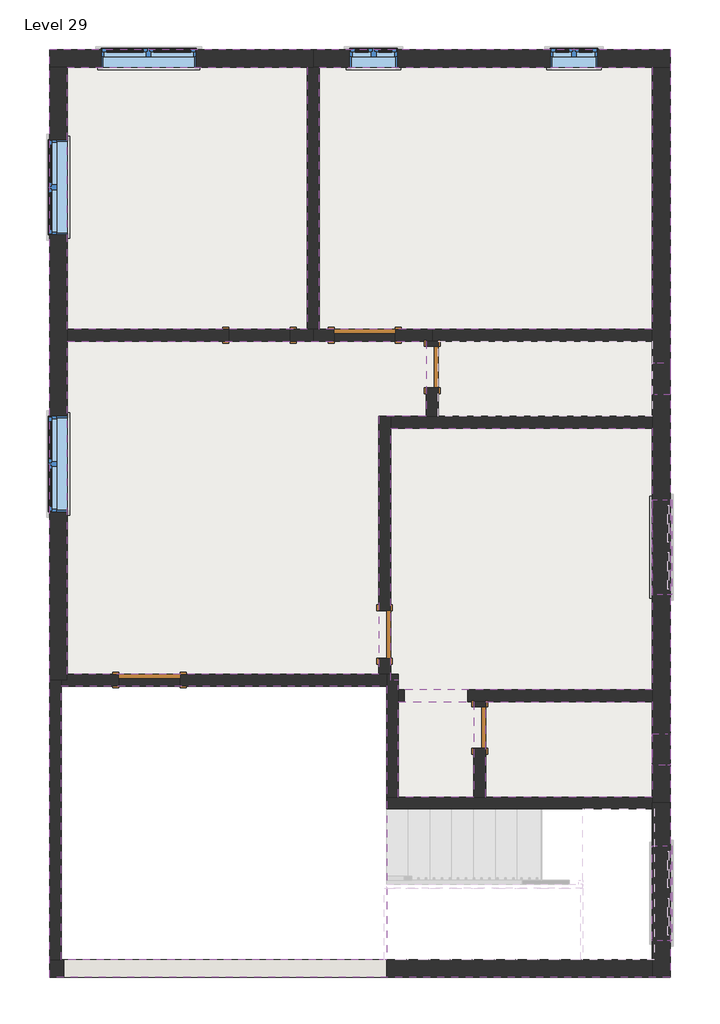
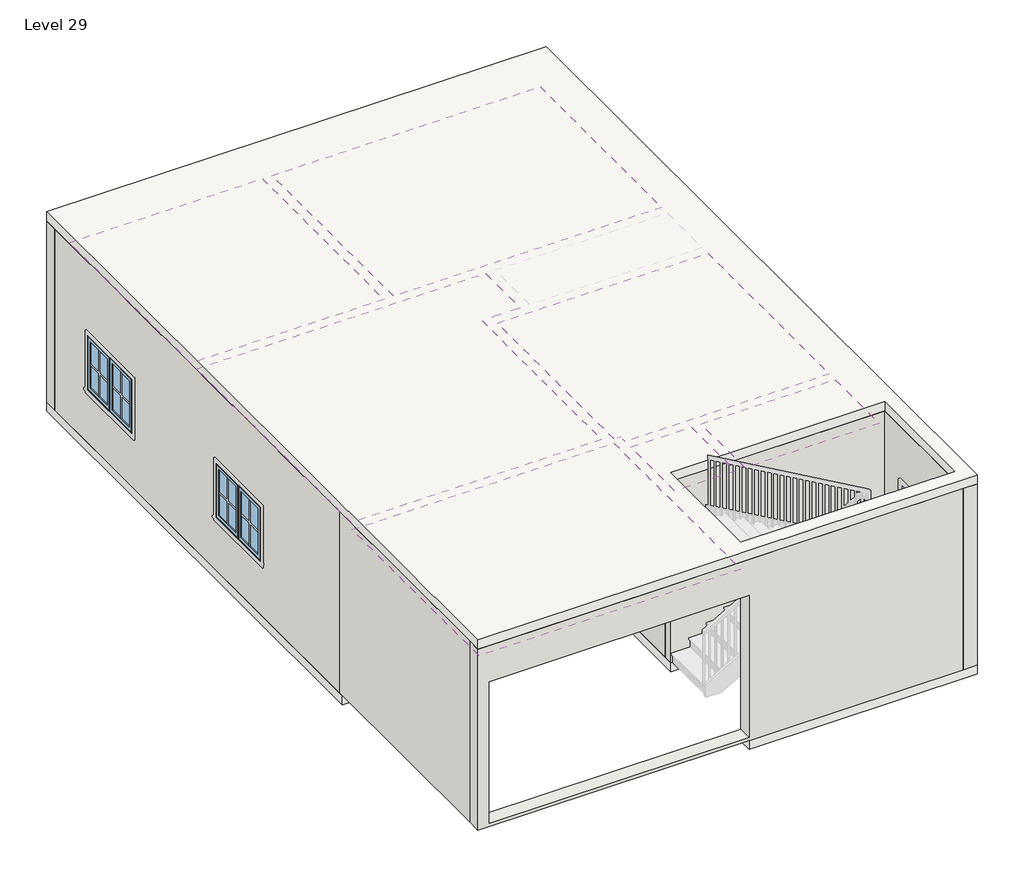
# One storey, part 1 of 2: 27 walls, 13 windows, 7 coverings, 6 doors, 2 slabs.
"""IFC4 building model written with IfcOpenShell, lengths in millimetres."""

from ifc_helpers import new_model, si_unit, frame, origin, place, context, project, spatial, polyline, outline, extrude, faceted_brep, transform, mapped, element, save
from components import door_2908be75, door_9ea4ff49, door_dc34e247, door_b804d09e, fixed_2_415b3208, window_casement_double_3_c417fced, window_casement_double_4_c19c33cb

model = new_model("IFC4")

# Units and contexts
model_context = context("Model", 3, world=origin())
ifc_project = project(units=[si_unit("LENGTHUNIT", "METRE", prefix="MILLI")], contexts=[model_context])

# Site, building, storey
site = spatial("IfcSite", under=ifc_project)
building = spatial("IfcBuilding", under=site)
storey = spatial("IfcBuildingStorey", under=building, Name="Level 29", Elevation=25603.2)

# Coverings
placement = place(None, origin())
element("IfcCovering", 1, ObjectType="2' x 4' ACT System", at=placement, inside=storey, context=model_context, shape_type="SweptSolid", body=[
    extrude(outline(polyline([(-5680.5154463, 2323.8455275), (-5680.5154463, 5678.2330275), (-2607.1154463, 5678.2330275), (-2607.1154463, 2323.8455275), (-5680.5154463, 2323.8455275)])), frame((0.0, 0.0, 28346.4), z_axis=(0.0, 0.0, 1.0), x_axis=(1.0, 0.0, 0.0)), (0.0, 0.0, 1.0), 57.15),
])
element("IfcCovering", 2, ObjectType="2' x 4' ACT System", at=placement, inside=storey, context=model_context, shape_type="SweptSolid", body=[
    extrude(outline(polyline([(-2454.7154463, 2323.8455275), (-2454.7154463, 5678.2330275), (1812.4845537, 5678.2330275), (1812.4845537, 2323.8455275), (-2454.7154463, 2323.8455275)])), frame((0.0, 0.0, 28346.4), z_axis=(0.0, 0.0, 1.0), x_axis=(1.0, 0.0, 0.0)), (0.0, 0.0, 1.0), 57.15),
])
element("IfcCovering", 3, ObjectType="2' x 4' ACT System", at=placement, inside=storey, context=model_context, shape_type="SweptSolid", body=[
    extrude(outline(polyline([(-5680.5154463, -2095.7544725), (-5680.5154463, 2171.4455275), (-1083.1154463, 2171.4455275), (-1083.1154463, 1206.2455275), (-1692.7154463, 1206.2455275), (-1692.7154463, -2095.7544725), (-5680.5154463, -2095.7544725)])), frame((0.0, 0.0, 28346.4), z_axis=(0.0, 0.0, 1.0), x_axis=(1.0, 0.0, 0.0)), (0.0, 0.0, 1.0), 57.15),
])
element("IfcCovering", 4, ObjectType="2' x 4' ACT System", at=placement, inside=storey, context=model_context, shape_type="SweptSolid", body=[
    extrude(outline(polyline([(1812.4845537, 1053.8455275), (1812.4845537, -2298.9544725), (-1438.7154463, -2298.9544725), (-1438.7154463, -2171.9544725), (-1540.3154463, -2171.9544725), (-1540.3154463, 1053.8455275), (1812.4845537, 1053.8455275)])), frame((0.0, 0.0, 28346.4), z_axis=(0.0, 0.0, 1.0), x_axis=(1.0, 0.0, 0.0)), (0.0, 0.0, 1.0), 57.15),
])
element("IfcCovering", 5, ObjectType="2' x 4' ACT System", at=placement, inside=storey, context=model_context, shape_type="SweptSolid", body=[
    extrude(outline(polyline([(1812.4845537, -2451.3544725), (1812.4845537, -3670.5544725), (-321.1154463, -3670.5544725), (-321.1154463, -2451.3544725), (1812.4845537, -2451.3544725)])), frame((0.0, 0.0, 28346.4), z_axis=(0.0, 0.0, 1.0), x_axis=(1.0, 0.0, 0.0)), (0.0, 0.0, 1.0), 57.15),
])
element("IfcCovering", 6, ObjectType="2' x 4' ACT System", at=placement, inside=storey, context=model_context, shape_type="SweptSolid", body=[
    extrude(outline(polyline([(-473.5154463, -2451.3544725), (-473.5154463, -3670.5544725), (-1438.7154463, -3670.5544725), (-1438.7154463, -2451.3544725), (-473.5154463, -2451.3544725)])), frame((0.0, 0.0, 28346.4), z_axis=(0.0, 0.0, 1.0), x_axis=(1.0, 0.0, 0.0)), (0.0, 0.0, 1.0), 57.15),
])
element("IfcCovering", 7, ObjectType="2' x 4' ACT System", at=placement, inside=storey, context=model_context, shape_type="SweptSolid", body=[
    extrude(outline(polyline([(-1591.1154463, -2248.1544725), (-1591.1154463, -5753.3544725), (-5756.7154463, -5753.3544725), (-5756.7154463, -2248.1544725), (-1591.1154463, -2248.1544725)])), frame((0.0, 0.0, 28346.4), z_axis=(0.0, 0.0, 1.0), x_axis=(1.0, 0.0, 0.0)), (0.0, 0.0, 1.0), 57.15),
])

# Doors
door_shape = door_2908be75(model_context)
element("IfcDoor", 8, ObjectType="Single-Flush : 1' 9\"", at=placement, inside=storey, context=model_context, shape_type="MappedRepresentation", body=[
    mapped(door_shape, transform((-397.3154463, -2781.5544725, 25603.2), x_axis=(0.0, 1.0, 0.0), y_axis=(-1.0, 0.0, 0.0), z_axis=(0.0, 0.0, 1.0))),
])
element("IfcDoor", 9, ObjectType="Single-Flush : 1' 9\"", at=placement, inside=storey, context=model_context, shape_type="MappedRepresentation", body=[
    mapped(door_shape, transform((-1006.9154463, 1841.2455275, 25603.2), x_axis=(0.0, 1.0, 0.0), y_axis=(-1.0, 0.0, 0.0), z_axis=(0.0, 0.0, 1.0))),
])
door_2_shape = door_9ea4ff49(model_context)
element("IfcDoor", 10, ObjectType="Single-Flush : 2'0\"", at=placement, inside=storey, context=model_context, shape_type="MappedRepresentation", body=[
    mapped(door_2_shape, transform((-1616.5154463, -1587.7544725, 25603.2), x_axis=(0.0, -1.0, 0.0), y_axis=(1.0, 0.0, 0.0), z_axis=(0.0, 0.0, 1.0))),
])
door_3_shape = door_dc34e247(model_context)
element("IfcDoor", 11, ObjectType="Single-Flush : 2'7\"", at=placement, inside=storey, context=model_context, shape_type="MappedRepresentation", body=[
    mapped(door_3_shape, transform((-4626.4154463, -2171.9544725, 25603.2), x_axis=(-1.0, 0.0, 0.0), y_axis=(0.0, -1.0, 0.0), z_axis=(0.0, 0.0, 1.0))),
])
element("IfcDoor", 12, ObjectType="Single-Flush : 2'7\"", at=placement, inside=storey, context=model_context, shape_type="MappedRepresentation", body=[
    mapped(door_3_shape, transform((-1870.5154463, 2247.6455275, 25603.2), x_axis=(-1.0, 0.0, 0.0), y_axis=(0.0, -1.0, 0.0), z_axis=(0.0, 0.0, 1.0))),
])
door_4_shape = door_b804d09e(model_context)
element("IfcDoor", 13, ObjectType="Single-Flush : 2'7\"", at=placement, inside=storey, context=model_context, shape_type="MappedRepresentation", body=[
    mapped(door_4_shape, transform((-3216.7154463, 2247.6455275, 25603.2), x_axis=(1.0, 0.0, 0.0), y_axis=(0.0, 1.0, 0.0), z_axis=(0.0, 0.0, 1.0))),
])

# Slabs
element("IfcSlab", 14, ObjectType="Generic - 6\"", at=placement, inside=storey, context=model_context, shape_type="SweptSolid", body=[
    extrude(outline(polyline([(-5909.1154463, -2248.1544725), (-5909.1154463, 5906.8330275), (2041.0845537, 5906.8330275), (2041.0845537, -5981.9544725), (-1591.1154463, -5981.9544725), (-1591.1154463, -5753.3544725), (1812.4845537, -5753.3544725), (1812.4845537, -3822.9544725), (-1591.1154463, -3822.9544725), (-1591.1154463, -2248.1544725), (-5756.7154463, -2248.1544725), (-5909.1154463, -2248.1544725)])), frame((0.0, 0.0, 25450.8), z_axis=(0.0, 0.0, 1.0), x_axis=(1.0, 0.0, 0.0)), (0.0, 0.0, 1.0), 152.4),
])
element("IfcSlab", 15, ObjectType="Generic - 6\"", at=placement, inside=storey, context=model_context, shape_type="SweptSolid", body=[
    extrude(outline(polyline([(2041.0845537, 5906.8330275), (2041.0845537, -5981.9544725), (-5909.1154463, -5981.9544725), (-5909.1154463, 5906.8330275), (2041.0845537, 5906.8330275)]), holes=[polyline([(1812.4845537, -3822.9544725), (-1591.1154463, -3822.9544725), (-1591.1154463, -5753.3544725), (1812.4845537, -5753.3544725), (1812.4845537, -3822.9544725)])]), frame((0.0, 0.0, 28651.2), z_axis=(0.0, 0.0, 1.0), x_axis=(1.0, 0.0, 0.0)), (0.0, 0.0, 1.0), 152.4),
])

# Walls
element("IfcWall", 16, ObjectType="Generic - 6\"", at=placement, inside=storey, context=model_context, shape_type="Brep", body=[
    faceted_brep([(-5909.1154463, -2171.9544725, 25603.2), (-5909.1154463, -5753.3544725, 25603.2), (-5909.1154463, -5753.3544725, 28651.2), (-5909.1154463, -2171.9544725, 28651.2), (-5756.7154463, -2171.9544725, 25603.2), (-5756.7154463, -2171.9544725, 28651.2), (-5756.7154463, -2248.1544725, 28651.2), (-5756.7154463, -5753.3544725, 28651.2), (-5756.7154463, -5753.3544725, 25603.2), (-5756.7154463, -2248.1544725, 25603.2)], [[[0, 1, 2, 3]], [[4, 5, 6, 7, 8, 9]], [[1, 0, 4, 9, 8]], [[3, 2, 7, 6, 5]], [[0, 3, 5, 4]], [[2, 1, 8, 7]]]),
])
element("IfcWall", 17, ObjectType="Generic - 6\"", at=placement, inside=storey, context=model_context, shape_type="Brep", body=[
    faceted_brep([(1812.4845537, -3670.5544725, 25603.2), (-321.1154463, -3670.5544725, 25603.2), (-473.5154463, -3670.5544725, 25603.2), (-1438.7154463, -3670.5544725, 25603.2), (-1591.1154463, -3670.5544725, 25603.2), (-1591.1154463, -3670.5544725, 28651.2), (-1438.7154463, -3670.5544725, 28651.2), (-473.5154463, -3670.5544725, 28651.2), (-321.1154463, -3670.5544725, 28651.2), (1812.4845537, -3670.5544725, 28651.2), (1812.4845537, -3822.9544725, 25603.2), (1812.4845537, -3822.9544725, 28651.2), (-1591.1154463, -3822.9544725, 28651.2), (-1591.1154463, -3822.9544725, 25603.2), (1812.4845537, -3746.7544725, 25603.2), (1812.4845537, -3746.7544725, 28651.2)], [[[0, 1, 2, 3, 4, 5, 6, 7, 8, 9]], [[10, 11, 12, 13]], [[4, 3, 2, 1, 0, 14, 10, 13]], [[9, 8, 7, 6, 5, 12, 11, 15]], [[5, 4, 13, 12]], [[0, 9, 15, 11, 10, 14]]]),
])
element("IfcWall", 18, ObjectType="Generic - 6\"", at=placement, inside=storey, context=model_context, shape_type="Brep", body=[
    faceted_brep([(-1438.7154463, -3670.5544725, 25603.2), (-1438.7154463, -2451.3544725, 25603.2), (-1438.7154463, -2298.9544725, 25603.2), (-1438.7154463, -2095.7544725, 25603.2), (-1438.7154463, -2095.7544725, 28651.2), (-1438.7154463, -2298.9544725, 28651.2), (-1438.7154463, -2451.3544725, 28651.2), (-1438.7154463, -3670.5544725, 28651.2), (-1591.1154463, -3670.5544725, 25603.2), (-1591.1154463, -3670.5544725, 28651.2), (-1591.1154463, -2248.1544725, 28651.2), (-1591.1154463, -2171.9544725, 28651.2), (-1591.1154463, -2095.7544725, 28651.2), (-1591.1154463, -2095.7544725, 25603.2), (-1591.1154463, -2171.9544725, 25603.2), (-1591.1154463, -2248.1544725, 25603.2), (-1540.3154463, -2095.7544725, 25603.2), (-1540.3154463, -2095.7544725, 28651.2)], [[[0, 1, 2, 3, 4, 5, 6, 7]], [[8, 9, 10, 11, 12, 13, 14, 15]], [[3, 2, 1, 0, 8, 15, 14, 13, 16]], [[7, 6, 5, 4, 17, 12, 11, 10, 9]], [[0, 7, 9, 8]], [[4, 3, 16, 13, 12, 17]]]),
])
element("IfcWall", 19, ObjectType="Generic - 6\"", at=placement, inside=storey, context=model_context, shape_type="Brep", body=[
    faceted_brep([(-5020.1154463, -2095.7544725, 27736.8), (-5020.1154463, -2095.7544725, 25603.2), (-5680.5154463, -2095.7544725, 25603.2), (-5680.5154463, -2095.7544725, 28651.2), (-1692.7154463, -2095.7544725, 28651.2), (-1591.1154463, -2095.7544725, 28651.2), (-1591.1154463, -2095.7544725, 25603.2), (-1692.7154463, -2095.7544725, 25603.2), (-4232.7154463, -2095.7544725, 25603.2), (-4232.7154463, -2095.7544725, 27736.8), (-5756.7154463, -2248.1544725, 25603.2), (-5020.1154463, -2248.1544725, 25603.2), (-5020.1154463, -2248.1544725, 27736.8), (-4232.7154463, -2248.1544725, 27736.8), (-4232.7154463, -2248.1544725, 25603.2), (-1591.1154463, -2248.1544725, 25603.2), (-1591.1154463, -2248.1544725, 28651.2), (-5756.7154463, -2248.1544725, 28651.2), (-5756.7154463, -2171.9544725, 25603.2), (-5680.5154463, -2171.9544725, 25603.2), (-5680.5154463, -2171.9544725, 28651.2), (-5756.7154463, -2171.9544725, 28651.2)], [[[0, 1, 2, 3, 4, 5, 6, 7, 8, 9]], [[10, 11, 12, 13, 14, 15, 16, 17]], [[2, 1, 11, 10, 18, 19]], [[8, 7, 6, 15, 14]], [[5, 4, 3, 20, 21, 17, 16]], [[3, 2, 19, 20]], [[19, 18, 21, 20]], [[18, 10, 17, 21]], [[6, 5, 16, 15]], [[12, 11, 1, 0]], [[13, 12, 0, 9]], [[14, 13, 9, 8]]]),
])
element("IfcWall", 20, ObjectType="Generic - 6\"", at=placement, inside=storey, context=model_context, shape_type="Brep", body=[
    faceted_brep([(1812.4845537, -2451.3544725, 25603.2), (1812.4845537, -2451.3544725, 28651.2), (-321.1154463, -2451.3544725, 28651.2), (-473.5154463, -2451.3544725, 28651.2), (-1438.7154463, -2451.3544725, 28651.2), (-1438.7154463, -2451.3544725, 25603.2), (-1367.0206652, -2451.3544725, 25603.2), (-1367.0206652, -2451.3544725, 28041.6), (-547.4818767, -2451.3544725, 28041.6), (-547.4818767, -2451.3544725, 25603.2), (-473.5154463, -2451.3544725, 25603.2), (-321.1154463, -2451.3544725, 25603.2), (1812.4845537, -2298.9544725, 28651.2), (1812.4845537, -2298.9544725, 25603.2), (-547.4818767, -2298.9544725, 25603.2), (-547.4818767, -2298.9544725, 28041.6), (-1367.0206652, -2298.9544725, 28041.6), (-1367.0206652, -2298.9544725, 25603.2), (-1438.7154463, -2298.9544725, 25603.2), (-1438.7154463, -2298.9544725, 28651.2)], [[[0, 1, 2, 3, 4, 5, 6, 7, 8, 9, 10, 11]], [[12, 13, 14, 15, 16, 17, 18, 19]], [[5, 18, 17, 6]], [[13, 0, 11, 10, 9, 14]], [[4, 3, 2, 1, 12, 19]], [[1, 0, 13, 12]], [[5, 4, 19, 18]], [[7, 16, 15, 8]], [[16, 7, 6, 17]], [[8, 15, 14, 9]]]),
])
element("IfcWall", 21, ObjectType="Generic - 6\"", at=placement, inside=storey, context=model_context, shape_type="SweptSolid", body=[
    extrude(outline(polyline([(-2451.3544725, 25603.2), (-2514.8544725, 25603.2), (-2514.8544725, 27736.8), (-3048.2544725, 27736.8), (-3048.2544725, 25603.2), (-3670.5544725, 25603.2), (-3670.5544725, 28651.2), (-2451.3544725, 28651.2), (-2451.3544725, 25603.2)])), frame((-473.5154463, 0.0, 0.0), z_axis=(1.0, 0.0, 0.0), x_axis=(0.0, 1.0, 0.0)), (0.0, 0.0, 1.0), 152.4),
])
element("IfcWall", 22, ObjectType="Generic - 6\"", at=placement, inside=storey, context=model_context, shape_type="Brep", body=[
    faceted_brep([(-1540.3154463, -2095.7544725, 25603.2), (-1540.3154463, -1892.5544725, 25603.2), (-1540.3154463, -1892.5544725, 27736.8), (-1540.3154463, -1282.9544725, 27736.8), (-1540.3154463, -1282.9544725, 25603.2), (-1540.3154463, 1053.8455275, 25603.2), (-1540.3154463, 1206.2455275, 25603.2), (-1540.3154463, 1206.2455275, 28651.2), (-1540.3154463, 1053.8455275, 28651.2), (-1540.3154463, -2095.7544725, 28651.2), (-1692.7154463, -1892.5544725, 27736.8), (-1692.7154463, -1892.5544725, 25603.2), (-1692.7154463, -2095.7544725, 25603.2), (-1692.7154463, -2095.7544725, 28651.2), (-1692.7154463, 1206.2455275, 28651.2), (-1692.7154463, 1206.2455275, 25603.2), (-1692.7154463, -1282.9544725, 25603.2), (-1692.7154463, -1282.9544725, 27736.8), (-1591.1154463, -2095.7544725, 25603.2), (-1591.1154463, -2095.7544725, 28651.2)], [[[0, 1, 2, 3, 4, 5, 6, 7, 8, 9]], [[10, 11, 12, 13, 14, 15, 16, 17]], [[16, 15, 6, 5, 4]], [[12, 11, 1, 0, 18]], [[9, 8, 7, 14, 13, 19]], [[0, 9, 19, 13, 12, 18]], [[7, 6, 15, 14]], [[2, 1, 11, 10]], [[3, 2, 10, 17]], [[4, 3, 17, 16]]]),
])
element("IfcWall", 23, ObjectType="Generic - 6\"", at=placement, inside=storey, context=model_context, shape_type="Brep", body=[
    faceted_brep([(-1540.3154463, 1053.8455275, 25603.2), (1812.4845537, 1053.8455275, 25603.2), (1812.4845537, 1053.8455275, 28651.2), (-1540.3154463, 1053.8455275, 28651.2), (-1540.3154463, 1206.2455275, 25603.2), (-1540.3154463, 1206.2455275, 28651.2), (-1083.1154463, 1206.2455275, 28651.2), (-930.7154463, 1206.2455275, 28651.2), (1812.4845537, 1206.2455275, 28651.2), (1812.4845537, 1206.2455275, 25603.2), (-930.7154463, 1206.2455275, 25603.2), (-1083.1154463, 1206.2455275, 25603.2)], [[[0, 1, 2, 3]], [[4, 5, 6, 7, 8, 9, 10, 11]], [[1, 0, 4, 11, 10, 9]], [[3, 2, 8, 7, 6, 5]], [[0, 3, 5, 4]], [[2, 1, 9, 8]]]),
])
element("IfcWall", 24, ObjectType="Generic - 6\"", at=placement, inside=storey, context=model_context, shape_type="Brep", body=[
    faceted_brep([(-930.7154463, 2107.9455275, 27736.8), (-930.7154463, 2107.9455275, 25603.2), (-930.7154463, 2171.4455275, 25603.2), (-930.7154463, 2171.4455275, 28651.2), (-930.7154463, 1206.2455275, 28651.2), (-930.7154463, 1206.2455275, 25603.2), (-930.7154463, 1574.5455275, 25603.2), (-930.7154463, 1574.5455275, 27736.8), (-1083.1154463, 2171.4455275, 25603.2), (-1083.1154463, 2107.9455275, 25603.2), (-1083.1154463, 2107.9455275, 27736.8), (-1083.1154463, 1574.5455275, 27736.8), (-1083.1154463, 1574.5455275, 25603.2), (-1083.1154463, 1206.2455275, 25603.2), (-1083.1154463, 1206.2455275, 28651.2), (-1083.1154463, 2171.4455275, 28651.2), (-1006.9154463, 2171.4455275, 25603.2), (-1006.9154463, 2171.4455275, 28651.2)], [[[0, 1, 2, 3, 4, 5, 6, 7]], [[8, 9, 10, 11, 12, 13, 14, 15]], [[6, 5, 13, 12]], [[2, 1, 9, 8, 16]], [[4, 3, 17, 15, 14]], [[5, 4, 14, 13]], [[10, 9, 1, 0]], [[11, 10, 0, 7]], [[12, 11, 7, 6]], [[3, 2, 16, 8, 15, 17]]]),
])
element("IfcWall", 25, ObjectType="Generic - 6\"", at=placement, inside=storey, context=model_context, shape_type="Brep", body=[
    faceted_brep([(1812.4845537, 2323.8455275, 25603.2), (-1006.9154463, 2323.8455275, 25603.2), (-1006.9154463, 2323.8455275, 28651.2), (1812.4845537, 2323.8455275, 28651.2), (1812.4845537, 2171.4455275, 25603.2), (1812.4845537, 2171.4455275, 28651.2), (-930.7154463, 2171.4455275, 28651.2), (-1006.9154463, 2171.4455275, 28651.2), (-1006.9154463, 2171.4455275, 25603.2), (-930.7154463, 2171.4455275, 25603.2)], [[[0, 1, 2, 3]], [[4, 5, 6, 7, 8, 9]], [[1, 0, 4, 9, 8]], [[2, 1, 8, 7]], [[3, 2, 7, 6, 5]], [[0, 3, 5, 4]]]),
])
element("IfcWall", 26, ObjectType="Generic - 6\"", at=placement, inside=storey, context=model_context, shape_type="Brep", body=[
    faceted_brep([(-2607.1154463, 5678.2330275, 25603.2), (-2607.1154463, 2323.8455275, 25603.2), (-2607.1154463, 2323.8455275, 28651.2), (-2607.1154463, 5678.2330275, 28651.2), (-2454.7154463, 5678.2330275, 25603.2), (-2454.7154463, 5678.2330275, 28651.2), (-2454.7154463, 2323.8455275, 28651.2), (-2454.7154463, 2323.8455275, 25603.2), (-2530.9154463, 5678.2330275, 25603.2), (-2530.9154463, 2323.8455275, 25603.2), (-2530.9154463, 2323.8455275, 28651.2), (-2530.9154463, 5678.2330275, 28651.2)], [[[0, 1, 2, 3]], [[4, 5, 6, 7]], [[1, 0, 8, 4, 7, 9]], [[3, 2, 10, 6, 5, 11]], [[0, 3, 11, 5, 4, 8]], [[2, 1, 9, 7, 6, 10]]]),
])
element("IfcWall", 27, ObjectType="Generic - 6\"", at=placement, inside=storey, context=model_context, shape_type="Brep", body=[
    faceted_brep([(-2530.9154463, 2323.8455275, 25603.2), (-2607.1154463, 2323.8455275, 25603.2), (-2823.0154463, 2323.8455275, 25603.2), (-2823.0154463, 2323.8455275, 27736.8), (-3610.4154463, 2323.8455275, 27736.8), (-3610.4154463, 2323.8455275, 25603.2), (-5680.5154463, 2323.8455275, 25603.2), (-5680.5154463, 2323.8455275, 28651.2), (-2607.1154463, 2323.8455275, 28651.2), (-2530.9154463, 2323.8455275, 28651.2), (-2823.0154463, 2171.4455275, 27736.8), (-2823.0154463, 2171.4455275, 25603.2), (-2530.9154463, 2171.4455275, 25603.2), (-2530.9154463, 2171.4455275, 28651.2), (-5680.5154463, 2171.4455275, 28651.2), (-5680.5154463, 2171.4455275, 25603.2), (-3610.4154463, 2171.4455275, 25603.2), (-3610.4154463, 2171.4455275, 27736.8)], [[[0, 1, 2, 3, 4, 5, 6, 7, 8, 9]], [[10, 11, 12, 13, 14, 15, 16, 17]], [[16, 15, 6, 5]], [[12, 11, 2, 1, 0]], [[9, 8, 7, 14, 13]], [[0, 9, 13, 12]], [[7, 6, 15, 14]], [[5, 4, 17, 16]], [[4, 3, 10, 17]], [[3, 2, 11, 10]]]),
])
element("IfcWall", 28, ObjectType="Generic - 6\"", at=placement, inside=storey, context=model_context, shape_type="Brep", body=[
    faceted_brep([(-2264.2154463, 2323.8455275, 27736.8), (-2264.2154463, 2323.8455275, 25603.2), (-2454.7154463, 2323.8455275, 25603.2), (-2530.9154463, 2323.8455275, 25603.2), (-2530.9154463, 2323.8455275, 28651.2), (-2454.7154463, 2323.8455275, 28651.2), (-1006.9154463, 2323.8455275, 28651.2), (-1006.9154463, 2323.8455275, 25603.2), (-1476.8154463, 2323.8455275, 25603.2), (-1476.8154463, 2323.8455275, 27736.8), (-2530.9154463, 2171.4455275, 25603.2), (-2264.2154463, 2171.4455275, 25603.2), (-2264.2154463, 2171.4455275, 27736.8), (-1476.8154463, 2171.4455275, 27736.8), (-1476.8154463, 2171.4455275, 25603.2), (-1083.1154463, 2171.4455275, 25603.2), (-1006.9154463, 2171.4455275, 25603.2), (-1006.9154463, 2171.4455275, 28651.2), (-1083.1154463, 2171.4455275, 28651.2), (-2530.9154463, 2171.4455275, 28651.2)], [[[0, 1, 2, 3, 4, 5, 6, 7, 8, 9]], [[10, 11, 12, 13, 14, 15, 16, 17, 18, 19]], [[8, 7, 16, 15, 14]], [[3, 2, 1, 11, 10]], [[4, 3, 10, 19]], [[6, 5, 4, 19, 18, 17]], [[7, 6, 17, 16]], [[14, 13, 9, 8]], [[13, 12, 0, 9]], [[12, 11, 1, 0]]]),
])
element("IfcWall", 29, ObjectType="Generic - 6\"", at=placement, inside=storey, context=model_context, shape_type="SweptSolid", body=[
    extrude(outline(polyline([(-5680.5154463, -2095.7544725), (-1692.7154463, -2095.7544725), (-1692.7154463, -2171.9544725), (-1591.1154463, -2171.9544725), (-1591.1154463, -2248.1544725), (-5756.7154463, -2248.1544725), (-5756.7154463, -2171.9544725), (-5680.5154463, -2171.9544725), (-5680.5154463, -2095.7544725)])), frame((0.0, 0.0, 25603.2), z_axis=(0.0, 0.0, 1.0), x_axis=(1.0, 0.0, 0.0)), (0.0, 0.0, 1.0), 3048.0),
])
element("IfcWall", 30, ObjectType="Generic - 6\"", at=placement, inside=storey, context=model_context, shape_type="Brep", body=[
    faceted_brep([(-2607.1154463, 5678.2330275, 25603.2), (-2607.1154463, 2323.8455275, 25603.2), (-2607.1154463, 2323.8455275, 28651.2), (-2607.1154463, 5678.2330275, 28651.2), (-2454.7154463, 5678.2330275, 25603.2), (-2454.7154463, 5678.2330275, 28651.2), (-2454.7154463, 2323.8455275, 28651.2), (-2454.7154463, 2323.8455275, 25603.2), (-2530.9154463, 5678.2330275, 25603.2), (-2530.9154463, 2323.8455275, 25603.2), (-2530.9154463, 2323.8455275, 28651.2), (-2530.9154463, 5678.2330275, 28651.2)], [[[0, 1, 2, 3]], [[4, 5, 6, 7]], [[1, 0, 8, 4, 7, 9]], [[3, 2, 10, 6, 5, 11]], [[0, 3, 11, 5, 4, 8]], [[2, 1, 9, 7, 6, 10]]]),
])
element("IfcWall", 31, ObjectType="Generic - 6\"", at=placement, inside=storey, context=model_context, shape_type="Brep", body=[
    faceted_brep([(-2530.9154463, 2323.8455275, 25603.2), (-2607.1154463, 2323.8455275, 25603.2), (-5680.5154463, 2323.8455275, 25603.2), (-5680.5154463, 2323.8455275, 28651.2), (-2607.1154463, 2323.8455275, 28651.2), (-2530.9154463, 2323.8455275, 28651.2), (-2530.9154463, 2171.4455275, 25603.2), (-2530.9154463, 2171.4455275, 28651.2), (-5680.5154463, 2171.4455275, 28651.2), (-5680.5154463, 2171.4455275, 25603.2)], [[[0, 1, 2, 3, 4, 5]], [[6, 7, 8, 9]], [[2, 1, 0, 6, 9]], [[5, 4, 3, 8, 7]], [[0, 5, 7, 6]], [[3, 2, 9, 8]]]),
])
element("IfcWall", 32, ObjectType="Generic - 6\"", at=placement, inside=storey, context=model_context, shape_type="Brep", body=[
    faceted_brep([(-1006.9154463, 2323.8455275, 25603.2), (-2454.7154463, 2323.8455275, 25603.2), (-2530.9154463, 2323.8455275, 25603.2), (-2530.9154463, 2323.8455275, 28651.2), (-2454.7154463, 2323.8455275, 28651.2), (-1006.9154463, 2323.8455275, 28651.2), (-1006.9154463, 2171.4455275, 25603.2), (-1006.9154463, 2171.4455275, 28651.2), (-1083.1154463, 2171.4455275, 28651.2), (-2530.9154463, 2171.4455275, 28651.2), (-2530.9154463, 2171.4455275, 25603.2), (-1083.1154463, 2171.4455275, 25603.2)], [[[0, 1, 2, 3, 4, 5]], [[6, 7, 8, 9, 10, 11]], [[2, 1, 0, 6, 11, 10]], [[3, 2, 10, 9]], [[5, 4, 3, 9, 8, 7]], [[0, 5, 7, 6]]]),
])
element("IfcWall", 33, ObjectType="Generic - 9\"", at=placement, inside=storey, context=model_context, shape_type="Brep", body=[
    faceted_brep([(-5909.1154463, 5678.2330275, 25603.2), (-5680.5154463, 5678.2330275, 25603.2), (-2607.1154463, 5678.2330275, 25603.2), (-2530.9154463, 5678.2330275, 25603.2), (-2530.9154463, 5678.2330275, 28651.2), (-2607.1154463, 5678.2330275, 28651.2), (-5680.5154463, 5678.2330275, 28651.2), (-5909.1154463, 5678.2330275, 28651.2), (-4029.5154463, 5678.2330275, 27432.0), (-4029.5154463, 5678.2330275, 26517.6), (-5248.7154463, 5678.2330275, 26517.6), (-5248.7154463, 5678.2330275, 27432.0), (-5909.1154463, 5906.8330275, 25603.2), (-5909.1154463, 5906.8330275, 28651.2), (-2530.9154463, 5906.8330275, 28651.2), (-2530.9154463, 5906.8330275, 25603.2), (-4029.5154463, 5906.8330275, 27432.0), (-5248.7154463, 5906.8330275, 27432.0), (-5248.7154463, 5906.8330275, 26517.6), (-4029.5154463, 5906.8330275, 26517.6)], [[[0, 1, 2, 3, 4, 5, 6, 7], [8, 9, 10, 11]], [[12, 13, 14, 15], [16, 17, 18, 19]], [[3, 2, 1, 0, 12, 15]], [[4, 3, 15, 14]], [[7, 6, 5, 4, 14, 13]], [[0, 7, 13, 12]], [[9, 8, 16, 19]], [[10, 9, 19, 18]], [[11, 10, 18, 17]], [[8, 11, 17, 16]]]),
])
element("IfcWall", 34, ObjectType="Generic - 9\"", at=placement, inside=storey, context=model_context, shape_type="Brep", body=[
    faceted_brep([(1812.4845537, 5678.2330275, 25603.2), (1812.4845537, 2323.8455275, 25603.2), (1812.4845537, 2171.4455275, 25603.2), (1812.4845537, 1206.2455275, 25603.2), (1812.4845537, 1053.8455275, 25603.2), (1812.4845537, -2298.9544725, 25603.2), (1812.4845537, -2451.3544725, 25603.2), (1812.4845537, -3670.5544725, 25603.2), (1812.4845537, -3746.7544725, 25603.2), (1812.4845537, -3746.7544725, 28651.2), (1812.4845537, -3670.5544725, 28651.2), (1812.4845537, -2451.3544725, 28651.2), (1812.4845537, -2298.9544725, 28651.2), (1812.4845537, 1053.8455275, 28651.2), (1812.4845537, 1206.2455275, 28651.2), (1812.4845537, 2171.4455275, 28651.2), (1812.4845537, 2323.8455275, 28651.2), (1812.4845537, 5678.2330275, 28651.2), (1812.4845537, -1079.7544725, 27736.8), (1812.4845537, -1079.7544725, 26822.4), (1812.4845537, 139.4455275, 26822.4), (1812.4845537, 139.4455275, 27736.8), (1812.4845537, -3264.1544725, 28041.6), (1812.4845537, -3264.1544725, 27432.0), (1812.4845537, -2857.7544725, 27432.0), (1812.4845537, -2857.7544725, 28041.6), (1812.4845537, 1892.0455275, 28041.6), (1812.4845537, 1485.6455275, 28041.6), (1812.4845537, 1485.6455275, 27432.0), (1812.4845537, 1892.0455275, 27432.0), (2041.0845537, 5678.2330275, 25603.2), (2041.0845537, 5678.2330275, 28651.2), (2041.0845537, -3746.7544725, 28651.2), (2041.0845537, -3746.7544725, 25603.2), (2041.0845537, -1079.7544725, 27736.8), (2041.0845537, 139.4455275, 27736.8), (2041.0845537, 139.4455275, 26822.4), (2041.0845537, -1079.7544725, 26822.4), (2041.0845537, -3264.1544725, 28041.6), (2041.0845537, -2857.7544725, 28041.6), (2041.0845537, -2857.7544725, 27432.0), (2041.0845537, -3264.1544725, 27432.0), (2041.0845537, 1892.0455275, 28041.6), (2041.0845537, 1892.0455275, 27432.0), (2041.0845537, 1485.6455275, 27432.0), (2041.0845537, 1485.6455275, 28041.6)], [[[0, 1, 2, 3, 4, 5, 6, 7, 8, 9, 10, 11, 12, 13, 14, 15, 16, 17], [18, 19, 20, 21], [22, 23, 24, 25], [26, 27, 28, 29]], [[30, 31, 32, 33], [34, 35, 36, 37], [38, 39, 40, 41], [42, 43, 44, 45]], [[8, 7, 6, 5, 4, 3, 2, 1, 0, 30, 33]], [[9, 8, 33, 32]], [[17, 16, 15, 14, 13, 12, 11, 10, 9, 32, 31]], [[0, 17, 31, 30]], [[19, 18, 34, 37]], [[20, 19, 37, 36]], [[21, 20, 36, 35]], [[18, 21, 35, 34]], [[23, 22, 38, 41]], [[24, 23, 41, 40]], [[25, 24, 40, 39]], [[22, 25, 39, 38]], [[43, 42, 26, 29]], [[44, 43, 29, 28]], [[45, 44, 28, 27]], [[42, 45, 27, 26]]]),
])
element("IfcWall", 35, ObjectType="Generic - 9\"", at=placement, inside=storey, context=model_context, shape_type="Brep", body=[
    faceted_brep([(1812.4845537, -5753.3544725, 25603.2), (-5756.7154463, -5753.3544725, 25603.2), (-5909.1154463, -5753.3544725, 25603.2), (-5909.1154463, -5753.3544725, 28651.2), (-5756.7154463, -5753.3544725, 28651.2), (1812.4845537, -5753.3544725, 28651.2), (-1591.1154463, -5753.3544725, 28041.6), (-5729.1673724, -5753.3544725, 28041.6), (-5729.1673724, -5753.3544725, 25654.0), (-1591.1154463, -5753.3544725, 25654.0), (-5909.1154463, -5981.9544725, 25603.2), (1812.4845537, -5981.9544725, 25603.2), (1812.4845537, -5981.9544725, 28651.2), (-5909.1154463, -5981.9544725, 28651.2), (-5729.1673724, -5981.9544725, 28041.6), (-1591.1154463, -5981.9544725, 28041.6), (-1591.1154463, -5981.9544725, 25654.0), (-5729.1673724, -5981.9544725, 25654.0)], [[[0, 1, 2, 3, 4, 5], [6, 7, 8, 9]], [[10, 11, 12, 13], [14, 15, 16, 17]], [[2, 1, 0, 11, 10]], [[5, 4, 3, 13, 12]], [[0, 5, 12, 11]], [[6, 15, 14, 7]], [[8, 17, 16, 9]], [[15, 6, 9, 16]], [[7, 14, 17, 8]], [[3, 2, 10, 13]]]),
])
element("IfcWall", 36, ObjectType="Generic - 9\"", at=placement, inside=storey, context=model_context, shape_type="Brep", body=[
    faceted_brep([(-5909.1154463, 5678.2330275, 25603.2), (-5909.1154463, -2171.9544725, 25603.2), (-5909.1154463, -2171.9544725, 28651.2), (-5909.1154463, 5678.2330275, 28651.2), (-5909.1154463, 4751.1330275, 27432.0), (-5909.1154463, 3531.9330275, 27432.0), (-5909.1154463, 3531.9330275, 26517.6), (-5909.1154463, 4751.1330275, 26517.6), (-5909.1154463, 1206.2455275, 27432.0), (-5909.1154463, -12.9544725, 27432.0), (-5909.1154463, -12.9544725, 26517.6), (-5909.1154463, 1206.2455275, 26517.6), (-5680.5154463, 5678.2330275, 25603.2), (-5680.5154463, 5678.2330275, 28651.2), (-5680.5154463, 2323.8455275, 28651.2), (-5680.5154463, 2171.4455275, 28651.2), (-5680.5154463, -2095.7544725, 28651.2), (-5680.5154463, -2171.9544725, 28651.2), (-5680.5154463, -2171.9544725, 25603.2), (-5680.5154463, -2095.7544725, 25603.2), (-5680.5154463, 2171.4455275, 25603.2), (-5680.5154463, 2323.8455275, 25603.2), (-5680.5154463, 4751.1330275, 27432.0), (-5680.5154463, 4751.1330275, 26517.6), (-5680.5154463, 3531.9330275, 26517.6), (-5680.5154463, 3531.9330275, 27432.0), (-5680.5154463, 1206.2455275, 27432.0), (-5680.5154463, 1206.2455275, 26517.6), (-5680.5154463, -12.9544725, 26517.6), (-5680.5154463, -12.9544725, 27432.0), (-5756.7154463, -2171.9544725, 25603.2), (-5756.7154463, -2171.9544725, 28651.2)], [[[0, 1, 2, 3], [4, 5, 6, 7], [8, 9, 10, 11]], [[12, 13, 14, 15, 16, 17, 18, 19, 20, 21], [22, 23, 24, 25], [26, 27, 28, 29]], [[1, 0, 12, 21, 20, 19, 18, 30]], [[2, 1, 30, 18, 17, 31]], [[3, 2, 31, 17, 16, 15, 14, 13]], [[0, 3, 13, 12]], [[23, 22, 4, 7]], [[24, 23, 7, 6]], [[25, 24, 6, 5]], [[22, 25, 5, 4]], [[27, 26, 8, 11]], [[28, 27, 11, 10]], [[29, 28, 10, 9]], [[26, 29, 9, 8]]]),
])
element("IfcWall", 37, ObjectType="Generic - 9\"", at=placement, inside=storey, context=model_context, shape_type="Brep", body=[
    faceted_brep([(-2530.9154463, 5678.2330275, 25603.2), (-2454.7154463, 5678.2330275, 25603.2), (1812.4845537, 5678.2330275, 25603.2), (2041.0845537, 5678.2330275, 25603.2), (2041.0845537, 5678.2330275, 28651.2), (1812.4845537, 5678.2330275, 28651.2), (-2454.7154463, 5678.2330275, 28651.2), (-2530.9154463, 5678.2330275, 28651.2), (-1451.4154463, 5678.2330275, 27432.0), (-1451.4154463, 5678.2330275, 26517.6), (-2061.0154463, 5678.2330275, 26517.6), (-2061.0154463, 5678.2330275, 27432.0), (1113.9845537, 5678.2330275, 27432.0), (1113.9845537, 5678.2330275, 26517.6), (504.3845537, 5678.2330275, 26517.6), (504.3845537, 5678.2330275, 27432.0), (-2530.9154463, 5906.8330275, 25603.2), (-2530.9154463, 5906.8330275, 28651.2), (2041.0845537, 5906.8330275, 28651.2), (2041.0845537, 5906.8330275, 25603.2), (-1451.4154463, 5906.8330275, 27432.0), (-2061.0154463, 5906.8330275, 27432.0), (-2061.0154463, 5906.8330275, 26517.6), (-1451.4154463, 5906.8330275, 26517.6), (1113.9845537, 5906.8330275, 27432.0), (504.3845537, 5906.8330275, 27432.0), (504.3845537, 5906.8330275, 26517.6), (1113.9845537, 5906.8330275, 26517.6)], [[[0, 1, 2, 3, 4, 5, 6, 7], [8, 9, 10, 11], [12, 13, 14, 15]], [[16, 17, 18, 19], [20, 21, 22, 23], [24, 25, 26, 27]], [[3, 2, 1, 0, 16, 19]], [[7, 6, 5, 4, 18, 17]], [[0, 7, 17, 16]], [[4, 3, 19, 18]], [[8, 11, 21, 20]], [[11, 10, 22, 21]], [[10, 9, 23, 22]], [[9, 8, 20, 23]], [[12, 15, 25, 24]], [[15, 14, 26, 25]], [[14, 13, 27, 26]], [[13, 12, 24, 27]]]),
])
element("IfcWall", 38, ObjectType="Generic - 9\"", at=placement, inside=storey, context=model_context, shape_type="Brep", body=[
    faceted_brep([(1812.4845537, -3746.7544725, 25603.2), (1812.4845537, -3822.9544725, 25603.2), (1812.4845537, -5753.3544725, 25603.2), (1812.4845537, -5981.9544725, 25603.2), (1812.4845537, -5981.9544725, 28651.2), (1812.4845537, -5753.3544725, 28651.2), (1812.4845537, -3822.9544725, 28651.2), (1812.4845537, -3746.7544725, 28651.2), (1812.4845537, -5512.0544725, 27736.8), (1812.4845537, -5512.0544725, 26822.4), (1812.4845537, -4292.8544725, 26822.4), (1812.4845537, -4292.8544725, 27736.8), (2041.0845537, -3746.7544725, 25603.2), (2041.0845537, -3746.7544725, 28651.2), (2041.0845537, -5981.9544725, 28651.2), (2041.0845537, -5981.9544725, 25603.2), (2041.0845537, -5512.0544725, 27736.8), (2041.0845537, -4292.8544725, 27736.8), (2041.0845537, -4292.8544725, 26822.4), (2041.0845537, -5512.0544725, 26822.4)], [[[0, 1, 2, 3, 4, 5, 6, 7], [8, 9, 10, 11]], [[12, 13, 14, 15], [16, 17, 18, 19]], [[3, 2, 1, 0, 12, 15]], [[7, 6, 5, 4, 14, 13]], [[0, 7, 13, 12]], [[4, 3, 15, 14]], [[8, 11, 17, 16]], [[11, 10, 18, 17]], [[10, 9, 19, 18]], [[9, 8, 16, 19]]]),
])
element("IfcWall", 39, ObjectType="Generic - 9\"", at=placement, inside=storey, context=model_context, shape_type="SweptSolid", body=[
    extrude(outline(polyline([(25603.2, -5680.5154463), (25603.2, -2607.1154463), (28651.2, -2607.1154463), (28651.2, -5680.5154463), (25603.2, -5680.5154463)]), holes=[polyline([(27432.0, -4029.5154463), (26517.6, -4029.5154463), (26517.6, -5248.7154463), (27432.0, -5248.7154463), (27432.0, -4029.5154463)])]), frame((0.0, 5678.2330275, 0.0), z_axis=(0.0, 1.0, 0.0), x_axis=(0.0, 0.0, 1.0)), (0.0, 0.0, 1.0), 228.6),
])
element("IfcWall", 40, ObjectType="Generic - 9\"", at=placement, inside=storey, context=model_context, shape_type="Brep", body=[
    faceted_brep([(1812.4845537, -5753.3544725, 25603.2), (-5756.7154463, -5753.3544725, 25603.2), (-5909.1154463, -5753.3544725, 25603.2), (-5909.1154463, -5753.3544725, 28651.2), (-5756.7154463, -5753.3544725, 28651.2), (1812.4845537, -5753.3544725, 28651.2), (-1591.1154463, -5753.3544725, 28041.6), (-5729.1673724, -5753.3544725, 28041.6), (-5729.1673724, -5753.3544725, 25654.0), (-1591.1154463, -5753.3544725, 25654.0), (-5909.1154463, -5981.9544725, 25603.2), (1812.4845537, -5981.9544725, 25603.2), (1812.4845537, -5981.9544725, 28651.2), (-5909.1154463, -5981.9544725, 28651.2), (-5729.1673724, -5981.9544725, 28041.6), (-1591.1154463, -5981.9544725, 28041.6), (-1591.1154463, -5981.9544725, 25654.0), (-5729.1673724, -5981.9544725, 25654.0)], [[[0, 1, 2, 3, 4, 5], [6, 7, 8, 9]], [[10, 11, 12, 13], [14, 15, 16, 17]], [[2, 1, 0, 11, 10]], [[5, 4, 3, 13, 12]], [[6, 15, 14, 7]], [[8, 17, 16, 9]], [[15, 6, 9, 16]], [[7, 14, 17, 8]], [[3, 2, 10, 13]], [[0, 5, 12, 11]]]),
])
element("IfcWall", 41, ObjectType="Generic - 9\"", at=placement, inside=storey, context=model_context, shape_type="SweptSolid", body=[
    extrude(outline(polyline([(25603.2, -2454.7154463), (25603.2, 1812.4845537), (28651.2, 1812.4845537), (28651.2, -2454.7154463), (25603.2, -2454.7154463)]), holes=[polyline([(27432.0, -1451.4154463), (26517.6, -1451.4154463), (26517.6, -2061.0154463), (27432.0, -2061.0154463), (27432.0, -1451.4154463)]), polyline([(27432.0, 1113.9845537), (26517.6, 1113.9845537), (26517.6, 504.3845537), (27432.0, 504.3845537), (27432.0, 1113.9845537)])]), frame((0.0, 5678.2330275, 0.0), z_axis=(0.0, 1.0, 0.0), x_axis=(0.0, 0.0, 1.0)), (0.0, 0.0, 1.0), 228.6),
])
element("IfcWall", 42, ObjectType="Generic - 9\"", at=placement, inside=storey, context=model_context, shape_type="SweptSolid", body=[
    extrude(outline(polyline([(-3822.9544725, 25603.2), (-5753.3544725, 25603.2), (-5753.3544725, 28651.2), (-3822.9544725, 28651.2), (-3822.9544725, 25603.2)]), holes=[polyline([(-5512.0544725, 27736.8), (-5512.0544725, 26822.4), (-4292.8544725, 26822.4), (-4292.8544725, 27736.8), (-5512.0544725, 27736.8)])]), frame((1812.4845537, 0.0, 0.0), z_axis=(1.0, 0.0, 0.0), x_axis=(0.0, 1.0, 0.0)), (0.0, 0.0, 1.0), 228.6),
])

# Windows
fixed_2_shape = fixed_2_415b3208(model_context)
element("IfcWindow", 43, ObjectType="Fixed : 2'", at=placement, inside=storey, context=model_context, shape_type="MappedRepresentation", body=[
    mapped(fixed_2_shape, transform((1926.7845537, -3099.0544725, 27127.2), x_axis=(0.0, -1.0, 0.0), y_axis=(1.0, 0.0, 0.0), z_axis=(0.0, 0.0, 1.0))),
])
element("IfcWindow", 44, ObjectType="Fixed : 2'", at=placement, inside=storey, context=model_context, shape_type="MappedRepresentation", body=[
    mapped(fixed_2_shape, transform((1926.7845537, 1726.9455275, 27127.2), x_axis=(0.0, 1.0, 0.0), y_axis=(-1.0, 0.0, 0.0), z_axis=(0.0, 0.0, 1.0))),
])
window_casement_double_3_shape = window_casement_double_3_c417fced(model_context)
element("IfcWindow", 45, ObjectType="Window-Casement-Double : 3'", at=placement, inside=storey, context=model_context, shape_type="MappedRepresentation", body=[
    mapped(window_casement_double_3_shape, transform((-1756.2154463, 5792.5330275, 25603.2), x_axis=(1.0, 0.0, 0.0), y_axis=(0.0, 1.0, 0.0), z_axis=(0.0, 0.0, 1.0))),
])
element("IfcWindow", 46, ObjectType="Window-Casement-Double : 3'", at=placement, inside=storey, context=model_context, shape_type="MappedRepresentation", body=[
    mapped(window_casement_double_3_shape, transform((809.1845537, 5792.5330275, 25603.2), x_axis=(1.0, 0.0, 0.0), y_axis=(0.0, 1.0, 0.0), z_axis=(0.0, 0.0, 1.0))),
])
element("IfcWindow", 47, ObjectType="Window-Casement-Double : 3'", at=placement, inside=storey, context=model_context, shape_type="MappedRepresentation", body=[
    mapped(window_casement_double_3_shape, transform((-1756.2154463, 5792.5330275, 25603.2), x_axis=(1.0, 0.0, 0.0), y_axis=(0.0, 1.0, 0.0), z_axis=(0.0, 0.0, 1.0))),
])
element("IfcWindow", 48, ObjectType="Window-Casement-Double : 3'", at=placement, inside=storey, context=model_context, shape_type="MappedRepresentation", body=[
    mapped(window_casement_double_3_shape, transform((809.1845537, 5792.5330275, 25603.2), x_axis=(1.0, 0.0, 0.0), y_axis=(0.0, 1.0, 0.0), z_axis=(0.0, 0.0, 1.0))),
])
window_casement_double_4_shape = window_casement_double_4_c19c33cb(model_context)
element("IfcWindow", 49, ObjectType="Window-Casement-Double : 4'", at=placement, inside=storey, context=model_context, shape_type="MappedRepresentation", body=[
    mapped(window_casement_double_4_shape, transform((-4639.1154463, 5792.5330275, 25603.2), x_axis=(1.0, 0.0, 0.0), y_axis=(0.0, 1.0, 0.0), z_axis=(0.0, 0.0, 1.0))),
])
element("IfcWindow", 50, ObjectType="Window-Casement-Double : 4'", at=placement, inside=storey, context=model_context, shape_type="MappedRepresentation", body=[
    mapped(window_casement_double_4_shape, transform((-5794.8154463, 4141.5330275, 25603.2), x_axis=(0.0, 1.0, 0.0), y_axis=(-1.0, 0.0, 0.0), z_axis=(0.0, 0.0, 1.0))),
])
element("IfcWindow", 51, ObjectType="Window-Casement-Double : 4'", at=placement, inside=storey, context=model_context, shape_type="MappedRepresentation", body=[
    mapped(window_casement_double_4_shape, transform((-5794.8154463, 596.6455275, 25603.2), x_axis=(0.0, 1.0, 0.0), y_axis=(-1.0, 0.0, 0.0), z_axis=(0.0, 0.0, 1.0))),
])
element("IfcWindow", 52, ObjectType="Window-Casement-Double : 4'", at=placement, inside=storey, context=model_context, shape_type="MappedRepresentation", body=[
    mapped(window_casement_double_4_shape, transform((1926.7845537, -470.1544725, 25908.0), x_axis=(0.0, -1.0, 0.0), y_axis=(1.0, 0.0, 0.0), z_axis=(0.0, 0.0, 1.0))),
])
element("IfcWindow", 53, ObjectType="Window-Casement-Double : 4'", at=placement, inside=storey, context=model_context, shape_type="MappedRepresentation", body=[
    mapped(window_casement_double_4_shape, transform((1926.7845537, -4902.4544725, 25908.0), x_axis=(0.0, -1.0, 0.0), y_axis=(1.0, 0.0, 0.0), z_axis=(0.0, 0.0, 1.0))),
])
element("IfcWindow", 54, ObjectType="Window-Casement-Double : 4'", at=placement, inside=storey, context=model_context, shape_type="MappedRepresentation", body=[
    mapped(window_casement_double_4_shape, transform((-4639.1154463, 5792.5330275, 25603.2), x_axis=(1.0, 0.0, 0.0), y_axis=(0.0, 1.0, 0.0), z_axis=(0.0, 0.0, 1.0))),
])
element("IfcWindow", 55, ObjectType="Window-Casement-Double : 4'", at=placement, inside=storey, context=model_context, shape_type="MappedRepresentation", body=[
    mapped(window_casement_double_4_shape, transform((1926.7845537, -4902.4544725, 25908.0), x_axis=(0.0, -1.0, 0.0), y_axis=(1.0, 0.0, 0.0), z_axis=(0.0, 0.0, 1.0))),
])

save(model, "model.ifc")

# Revit data of these elements
# Type "2' x 4' ACT System"
#   Assembly Code = "C3030210"
#   built-in parameter 1002203 = 1 (stored number, unit not read)
#   built-in parameter 1002202 = 1 (stored number, unit not read)
#   Layers, outside or top first: 0' - 1 5/8" "Default" (function 1); 0' - 0 5/8" "Acoustic Ceiling Tile 24 x 48" (function 5)
# Type "Single-Flush : 1' 9\""
#   Type Mark = "10"
#   Construction Type Id = "MDOOR"
#   Assembly Code = "C1020"
#   Analytic Construction = "Metal"
#   Thickness = 0' - 2"
#   Heat Transfer Coefficient (U) = 0.651978 BTU/(h·ft²·°F)
#   Height = 7' - 0"
#   Trim Projection Ext = 0' - 1"
#   Trim Projection Int = 0' - 1"
#   Trim Width = 0' - 3"
#   Width = 1' - 9"
#   Define Thermal Properties by = 1
#   Door Material = Door - Panel
#   Frame Material = Door - Frame
#   Visual Light Transmittance = 0
#   Solar Heat Gain Coefficient = 0
#   Function = (empty or 0)
#   Wall Closure = (empty or 0)
# Type "Single-Flush : 2'0\""
#   Type Mark = "9"
#   Construction Type Id = "MDOOR"
#   Assembly Code = "C1020"
#   Analytic Construction = "Metal"
#   Thickness = 0' - 2"
#   Heat Transfer Coefficient (U) = 0.651978 BTU/(h·ft²·°F)
#   Height = 7' - 0"
#   Trim Projection Ext = 0' - 1"
#   Trim Projection Int = 0' - 1"
#   Trim Width = 0' - 3"
#   Width = 2' - 0"
#   Define Thermal Properties by = 1
#   Door Material = Door - Panel
#   Frame Material = Door - Frame
#   Visual Light Transmittance = 0
#   Solar Heat Gain Coefficient = 0
#   Function = (empty or 0)
#   Wall Closure = (empty or 0)
# Type "Single-Flush : 2'7\""
#   Type Mark = "8"
#   Construction Type Id = "MDOOR"
#   Assembly Code = "C1020"
#   Analytic Construction = "Metal"
#   Thickness = 0' - 2"
#   Heat Transfer Coefficient (U) = 0.651978 BTU/(h·ft²·°F)
#   Height = 7' - 0"
#   Trim Projection Ext = 0' - 1"
#   Trim Projection Int = 0' - 1"
#   Trim Width = 0' - 3"
#   Width = 2' - 7"
#   Define Thermal Properties by = 1
#   Door Material = Door - Panel
#   Frame Material = Door - Frame
#   Visual Light Transmittance = 0
#   Solar Heat Gain Coefficient = 0
#   Function = (empty or 0)
#   Wall Closure = (empty or 0)
# Type "Generic - 6\""
#   Assembly Code = "B1010"
#   Function = 0
#   Layers, outside or top first: 0' - 6" no material (function 1)
# Type "Generic - 6\""
#   Assembly Code = "B2010"
#   Layers, outside or top first: 0' - 6" no material (function 1)
# Type "Generic - 9\""
#   Assembly Code = "B2010"
#   Layers, outside or top first: 0' - 9" no material (function 1)
# Type "Fixed : 2'"
#   Type Mark = "20"
#   Construction Type Id = "GSP4R"
#   Assembly Code = "B2020100"
#   Analytic Construction = "1/8 in Pilkington single glazing"
#   Visual Light Transmittance = 0.9
#   Solar Heat Gain Coefficient = 0.78
#   Heat Transfer Coefficient (U) = 0.6496 BTU/(h·ft²·°F)
#   Height = 2' - 0"
#   Default Sill Height = 1' - 0"
#   Width = 1' - 4"
#   Window Inset = 0' - 0 3/4"
#   Define Thermal Properties by = 1
#   Glass Pane Material = Glass
#   Sash Material = Sash
#   Wall Closure = (empty or 0)
# Type "Window-Casement-Double : 3'"
#   Type Mark = "19"
#   Fire Rating = "0.5h"
#   Assembly Code = "B2020100"
#   Analytic Construction = "Double glazing - domestic"
#   Frame Extension [instance default] = 0' - 0 1/4"
#   Window Inset [instance default] = 0' - 0"
#   Wall Thickness [instance default] = 0' - 6"
#   Interior Wall Closure [instance default] = 0' - 2 1/4"
#   Half Width = 1' - 0"
#   Visual Light Transmittance = 0.81
#   Thermal Resistance (R) = 1.8146 (h·ft²·°F)/BTU
#   Solar Heat Gain Coefficient = 0.76
#   Rough Width = 2' - 0 1/2"
#   Rough Height = 3' - 0 1/2"
#   Height = 3' - 0"
#   Heat Transfer Coefficient (U) = 0.5511 BTU/(h·ft²·°F)
#   Exterior Wall Closure [instance default] = 0' - 1 1/4"
#   Extension Jamb [instance default] = 0' - 2 1/4"
#   Default Sill Height = 3' - 0"
#   Width = 2' - 0"
#   Muntin Visibility = yes
#   Interior Trim Visibility [instance default] = yes
#   Exterior Trim Visibility [instance default] = yes
#   Extension Jamb Visibility [instance default] = yes
#   Interior Trim Material = Wood - Stained
#   Muntin Pattern = Muntin Pattern_2x2 : Muntin Pattern_2x2
#   Interior Trim = Trim-Window-Interior-Flat : Picture Frame
#   Interior Frame Material = Wood - Stained
#   Glass Panel Material = Glass
#   Exterior Trim Material = Clad - White
#   Exterior Trim = Trim-Window-Exterior-Flat : with Sill
#   Exterior Frame Material = Clad - White
#   Wall Closure = (empty or 0)
# Type "Window-Casement-Double : 4'"
#   Type Mark = "18"
#   Fire Rating = "0.5h"
#   Assembly Code = "B2020100"
#   Analytic Construction = "Double glazing - domestic"
#   Frame Extension [instance default] = 0' - 0 1/4"
#   Window Inset [instance default] = 0' - 0"
#   Wall Thickness [instance default] = 0' - 6"
#   Interior Wall Closure [instance default] = 0' - 2 1/4"
#   Half Width = 2' - 0"
#   Visual Light Transmittance = 0.81
#   Thermal Resistance (R) = 1.8146 (h·ft²·°F)/BTU
#   Solar Heat Gain Coefficient = 0.76
#   Rough Width = 4' - 0 1/2"
#   Rough Height = 3' - 0 1/2"
#   Height = 3' - 0"
#   Heat Transfer Coefficient (U) = 0.5511 BTU/(h·ft²·°F)
#   Exterior Wall Closure [instance default] = 0' - 1 1/4"
#   Extension Jamb [instance default] = 0' - 2 1/4"
#   Default Sill Height = 3' - 0"
#   Width = 4' - 0"
#   Muntin Visibility = yes
#   Interior Trim Visibility [instance default] = yes
#   Exterior Trim Visibility [instance default] = yes
#   Extension Jamb Visibility [instance default] = yes
#   Interior Trim Material = Wood - Stained
#   Muntin Pattern = Muntin Pattern_2x2 : Muntin Pattern_2x2
#   Interior Trim = Trim-Window-Interior-Flat : Picture Frame
#   Interior Frame Material = Wood - Stained
#   Glass Panel Material = Glass
#   Exterior Trim Material = Clad - White
#   Exterior Trim = Trim-Window-Exterior-Flat : with Sill
#   Exterior Frame Material = Clad - White
#   Wall Closure = (empty or 0)
# Elements 1, 2, 3, 4, 5, 6, 7 (IfcCovering, "2' x 4' ACT System")
#   Height Offset From Level = 9' - 0"
#   Phase Created = New Construction
#   Materials on its faces: "Acoustic Ceiling Tile 24 x 48", "Default"
# Elements 8, 9 (IfcDoor, "Single-Flush : 1' 9\"")
#   Phase Created = New Construction
#   Materials on its faces: "Door - Frame", "Door - Panel"
# Element 10 (IfcDoor, "Single-Flush : 2'0\"")
#   Phase Created = New Construction
#   Materials on its faces: "Door - Frame", "Door - Panel"
# Elements 11, 12, 13 (IfcDoor, "Single-Flush : 2'7\"")
#   Phase Created = New Construction
#   Materials on its faces: "Door - Frame", "Door - Panel"
# Element 14 (IfcSlab, "Generic - 6\"")
#   built-in parameter 1001955 = -1.5708 (stored number, unit not read)
#   Height Offset From Level = 0' - 0"
#   Phase Created = New Construction
#   Materials on its faces: "Default Floor", "TILE"
# Element 15 (IfcSlab, "Generic - 6\"")
#   Height Offset From Level = 10' - 6"
#   Phase Created = New Construction
#   Materials on its faces: "Default Floor"
# Element 16 (IfcWall, "Generic - 6\"")
#   Top Offset = 0' - 0"
#   Base Offset = 0' - 0"
#   Unconnected Height = 10' - 0"
#   wall height = 10' - 0"
#   Phase Created = New Construction
#   Base Constraint = Level 29
#   Materials on its faces: "Default Wall", "WALL PAINT 4"
# Element 17 (IfcWall, "Generic - 6\"")
#   Top Offset = 0' - 0"
#   Base Offset = 0' - 0"
#   Unconnected Height = 10' - 0"
#   wall height = 10' - 0"
#   Phase Created = New Construction
#   Base Constraint = Level 29
#   Materials on its faces: "Default Wall", "MARBLE", "WALL PAINT 5"
# Element 18 (IfcWall, "Generic - 6\"")
#   Top Offset = 0' - 0"
#   Base Offset = 0' - 0"
#   Unconnected Height = 10' - 0"
#   wall height = 10' - 0"
#   Phase Created = New Construction
#   Base Constraint = Level 29
#   Materials on its faces: "Default Wall", "WALL PAINT 4", "MARBLE"
# Elements 19, 29 (IfcWall, "Generic - 6\"")
#   Top Offset = 0' - 0"
#   Base Offset = 0' - 0"
#   Unconnected Height = 10' - 0"
#   wall height = 10' - 0"
#   Phase Created = New Construction
#   Base Constraint = Level 29
#   Materials on its faces: "Default Wall", "WALL PAINT 2", "MARBLE"
# Elements 20, 23 (IfcWall, "Generic - 6\"")
#   Top Offset = 0' - 0"
#   Base Offset = 0' - 0"
#   Unconnected Height = 10' - 0"
#   wall height = 10' - 0"
#   Phase Created = New Construction
#   Base Constraint = Level 29
#   Materials on its faces: "Default Wall", "WALL PAINT 4", "WALL PAINT 5"
# Element 21 (IfcWall, "Generic - 6\"")
#   Top Offset = 0' - 0"
#   Base Offset = 0' - 0"
#   Unconnected Height = 10' - 0"
#   wall height = 10' - 0"
#   Phase Created = New Construction
#   Base Constraint = Level 29
#   Materials on its faces: "Default Wall", "WALL PAINT 5"
# Element 22 (IfcWall, "Generic - 6\"")
#   Top Offset = 0' - 0"
#   Base Offset = 0' - 0"
#   Unconnected Height = 10' - 0"
#   wall height = 10' - 0"
#   Phase Created = New Construction
#   Base Constraint = Level 29
#   Materials on its faces: "Default Wall", "WALL PAINT 4", "WALL PAINT 2", "WALL PAINT 5"
# Element 24 (IfcWall, "Generic - 6\"")
#   Top Offset = 0' - 0"
#   Base Offset = 0' - 0"
#   Unconnected Height = 10' - 0"
#   wall height = 10' - 0"
#   Phase Created = New Construction
#   Base Constraint = Level 29
#   Materials on its faces: "Default Wall", "WALL PAINT 5", "WALL PAINT 2"
# Element 25 (IfcWall, "Generic - 6\"")
#   Top Offset = 0' - 0"
#   Base Offset = 0' - 0"
#   Unconnected Height = 10' - 0"
#   wall height = 10' - 0"
#   Phase Created = New Construction
#   Base Constraint = Level 29
#   Materials on its faces: "Default Wall", "WALL PAINT 3", "WALL PAINT 5"
# Elements 26, 30 (IfcWall, "Generic - 6\"")
#   Top Offset = 0' - 0"
#   Base Offset = 0' - 0"
#   Unconnected Height = 10' - 0"
#   wall height = 10' - 0"
#   Phase Created = New Construction
#   Base Constraint = Level 29
#   Materials on its faces: "Default Wall", "WALL PAINT 1", "WALL PAINT 3"
# Elements 27, 31 (IfcWall, "Generic - 6\"")
#   Top Offset = 0' - 0"
#   Base Offset = 0' - 0"
#   Unconnected Height = 10' - 0"
#   wall height = 10' - 0"
#   Phase Created = New Construction
#   Base Constraint = Level 29
#   Materials on its faces: "Default Wall", "WALL PAINT 1", "WALL PAINT 2"
# Elements 28, 32 (IfcWall, "Generic - 6\"")
#   Top Offset = 0' - 0"
#   Base Offset = 0' - 0"
#   Unconnected Height = 10' - 0"
#   wall height = 10' - 0"
#   Phase Created = New Construction
#   Base Constraint = Level 29
#   Materials on its faces: "Default Wall", "WALL PAINT 3", "WALL PAINT 2"
# Elements 33, 39 (IfcWall, "Generic - 9\"")
#   Top Offset = 0' - 0"
#   Base Offset = 0' - 0"
#   Unconnected Height = 10' - 0"
#   wall height = 10' - 0"
#   Phase Created = New Construction
#   Base Constraint = Level 29
#   Materials on its faces: "Default Wall", "WALL PAINT 1"
# Elements 34, 36 (IfcWall, "Generic - 9\"")
#   Top Offset = 0' - 0"
#   Base Offset = 0' - 0"
#   Unconnected Height = 10' - 0"
#   wall height = 10' - 0"
#   Phase Created = New Construction
#   Base Constraint = Level 29
#   Materials on its faces: "Default Wall"
# Elements 35, 38, 40, 42 (IfcWall, "Generic - 9\"")
#   Top Offset = 0' - 0"
#   Base Offset = 0' - 0"
#   Unconnected Height = 10' - 0"
#   wall height = 10' - 0"
#   Phase Created = New Construction
#   Base Constraint = Level 29
#   Materials on its faces: "Default Wall", "WALL PAINT 4"
# Elements 37, 41 (IfcWall, "Generic - 9\"")
#   Top Offset = 0' - 0"
#   Base Offset = 0' - 0"
#   Unconnected Height = 10' - 0"
#   wall height = 10' - 0"
#   Phase Created = New Construction
#   Base Constraint = Level 29
#   Materials on its faces: "Default Wall", "WALL PAINT 3"
# Element 43 (IfcWindow, "Fixed : 2'")
#   Mark = "138"
#   Phase Created = New Construction
#   Materials on its faces: "Sash", "Glass"
# Element 44 (IfcWindow, "Fixed : 2'")
#   Mark = "139"
#   Phase Created = New Construction
#   Materials on its faces: "Sash", "Glass"
# Element 45 (IfcWindow, "Window-Casement-Double : 3'")
#   Mark = "136"
#   Window Inset = 0' - 0"
#   Interior Wall Closure = 0' - 2 1/4"
#   Frame Extension = 0' - 0 1/4"
#   Exterior Wall Closure = 0' - 1 1/4"
#   Interior Trim Visibility = yes
#   Exterior Trim Visibility = yes
#   Phase Created = New Construction
#   Materials on its faces: "Wood - Stained", "Glass", "Clad - White"
# Element 46 (IfcWindow, "Window-Casement-Double : 3'")
#   Mark = "137"
#   Window Inset = 0' - 0"
#   Interior Wall Closure = 0' - 2 1/4"
#   Frame Extension = 0' - 0 1/4"
#   Exterior Wall Closure = 0' - 1 1/4"
#   Interior Trim Visibility = yes
#   Exterior Trim Visibility = yes
#   Phase Created = New Construction
#   Materials on its faces: "Wood - Stained", "Glass", "Clad - White"
# Element 47 (IfcWindow, "Window-Casement-Double : 3'")
#   Mark = "142"
#   Window Inset = 0' - 0"
#   Interior Wall Closure = 0' - 2 1/4"
#   Frame Extension = 0' - 0 1/4"
#   Exterior Wall Closure = 0' - 1 1/4"
#   Interior Trim Visibility = yes
#   Exterior Trim Visibility = yes
#   Phase Created = New Construction
#   Materials on its faces: "Wood - Stained", "Glass", "Clad - White"
# Element 48 (IfcWindow, "Window-Casement-Double : 3'")
#   Mark = "143"
#   Window Inset = 0' - 0"
#   Interior Wall Closure = 0' - 2 1/4"
